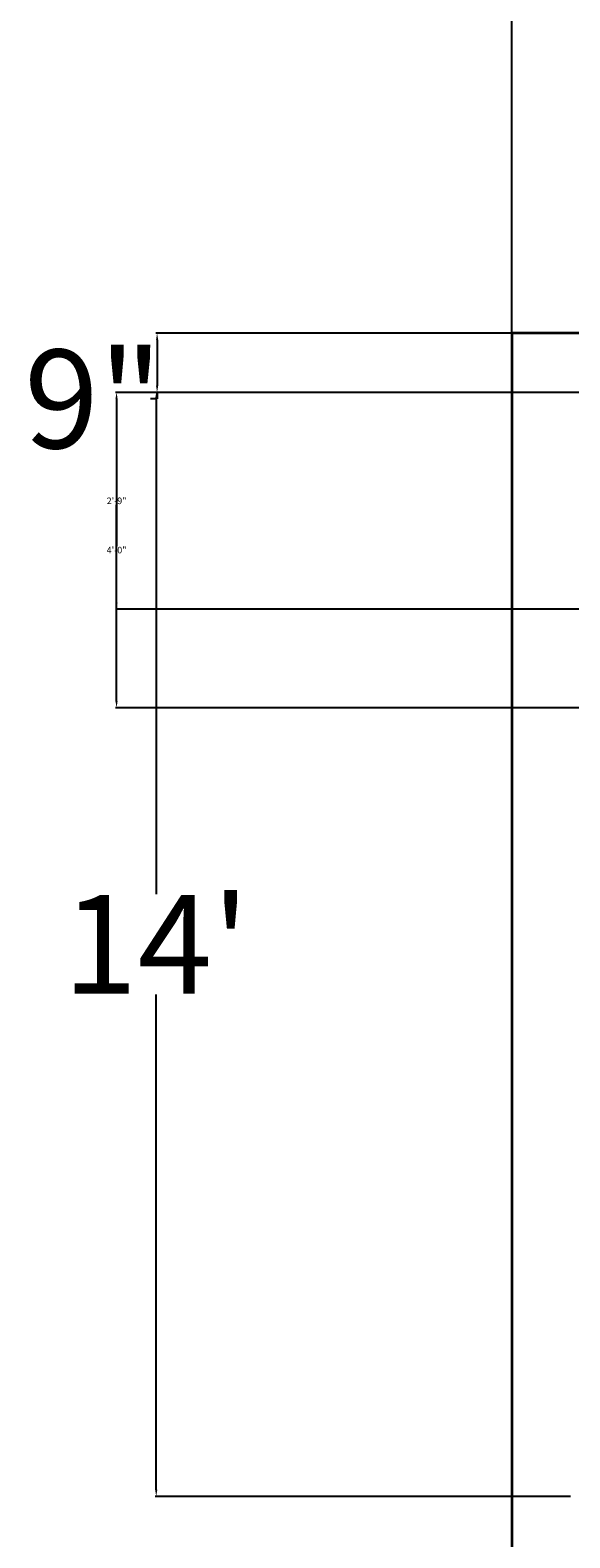
# Model space of a CAD drawing. Units: inches. Extents: x 371 to 1095, y -45 to 1219.
# Tile 14 of 18: x 419 to 502, y 799 to 1028. Entities that reach past the tile are written whole.
import ezdxf

# ---------------------------------------------------------------- set-up
doc = ezdxf.new("R2010")
doc.units = ezdxf.units.IN
doc.header["$MEASUREMENT"] = 0
doc.layers.add('A-ANNO-DIMS', color=2, linetype='Continuous', lineweight=18)
doc.layers.add('A-WALL', color=40, linetype='Continuous', lineweight=35)
doc.styles.get("Standard").update_dxf_attribs({"font": 'arial.ttf'})
doc.dimstyles.get("Standard").update_dxf_attribs({"dimtxt": 1, "dimasz": 1, "dimexe": 0.18, "dimexo": 0.0625, "dimgap": 0.09, "dimtad": 0, "dimtih": 1, "dimtoh": 1, "dimdec": 0, "dimzin": 0, "dimdsep": 46, "dimlunit": 3, "dimtxsty": 'Standard', "dimcen": 0.09, "dimadec": 0, "dimazin": 0, "dimtfac": 1, "dimtdec": 0, "dimtofl": 0, "dimtmove": 0, "dimatfit": 3, "dimfxl": 1, "dimtolj": 1, "dimtzin": 0, "dimarcsym": 0})

# ---------------------------------------------------------------- blocks, each defined once
blk = doc.blocks.new('*D8')
at = {"layer": 'A-ANNO-DIMS', "color": 0, "lineweight": -2, "transparency": 16777216}
for p, q in [((501.75, 973.03), (438.47, 973.03)), ((438.65, 972.03), (438.65, 896.65)), ((438.65, 806.03), (438.65, 881.4)), ((501.75, 805.03), (438.47, 805.03))]:
    blk.add_line(p, q, dxfattribs=at)
at = {"layer": 'A-ANNO-DIMS', "color": 0, "transparency": 16777216}
for points in [[(438.48, 972.03), (438.82, 972.03), (438.65, 973.03)], [(438.48, 806.03), (438.82, 806.03), (438.65, 805.03)]]:
    blk.add_solid(points, dxfattribs=at)
at = {"layer": 'Defpoints', "color": 0, "transparency": 16777216}
for p in [(501.81, 973.03), (438.65, 805.03), (501.81, 805.03)]:
    blk.add_point(p, dxfattribs=at)
at = {"layer": 'A-ANNO-DIMS', "color": 0, "transparency": 16777216, "insert": (438.65, 889.03), "char_height": 1, "attachment_point": 5}
blk.add_mtext("\\A1;{\\H15x;14'}", dxfattribs=at)
blk = doc.blocks.new('*D19')
at = {"layer": 'A-ANNO-DIMS', "color": 0, "lineweight": -2, "transparency": 16777216}
for p, q in [((501.75, 982.03), (438.6, 982.03)), ((438.78, 981.03), (438.78, 974.03)), ((501.75, 973.03), (438.6, 973.03)), ((438.78, 973.03), (438.78, 972.03)), ((438.78, 972.03), (437.78, 972.03))]:
    blk.add_line(p, q, dxfattribs=at)
at = {"layer": 'A-ANNO-DIMS', "color": 0, "transparency": 16777216}
for points in [[(438.62, 981.03), (438.95, 981.03), (438.78, 982.03)], [(438.62, 974.03), (438.95, 974.03), (438.78, 973.03)]]:
    blk.add_solid(points, dxfattribs=at)
at = {"layer": 'Defpoints', "color": 0, "transparency": 16777216}
for p in [(501.81, 982.03), (438.78, 973.03), (501.81, 973.03)]:
    blk.add_point(p, dxfattribs=at)
at = {"layer": 'A-ANNO-DIMS', "color": 0, "transparency": 16777216, "insert": (429.07, 972.03), "char_height": 1, "attachment_point": 5}
blk.add_mtext('\\A1;{\\H15x;9"}', dxfattribs=at)
blk = doc.blocks.new('*D50')
at = {"layer": 'A-ANNO-DIMS', "color": 0, "lineweight": -2, "transparency": 16777216}
for p, q in [((492.81, 982.09), (492.81, 1093.41)), ((493.81, 1093.23), (760.98, 1093.23)), ((1031.81, 1093.23), (764.64, 1093.23)), ((1032.81, 982.09), (1032.81, 1093.41))]:
    blk.add_line(p, q, dxfattribs=at)
at = {"layer": 'A-ANNO-DIMS', "color": 0, "transparency": 16777216}
for points in [[(493.81, 1093.39), (493.81, 1093.06), (492.81, 1093.23)], [(1031.81, 1093.39), (1031.81, 1093.06), (1032.81, 1093.23)]]:
    blk.add_solid(points, dxfattribs=at)
at = {"layer": 'Defpoints', "color": 0, "transparency": 16777216}
for p in [(1032.81, 1093.23), (492.81, 982.03), (1032.81, 982.03)]:
    blk.add_point(p, dxfattribs=at)
at = {"layer": 'A-ANNO-DIMS', "color": 0, "transparency": 16777216, "insert": (762.81, 1093.23), "char_height": 1, "attachment_point": 5}
blk.add_mtext('\\A1;45\'-0"', dxfattribs=at)
blk = doc.blocks.new('*D55')
at = {"layer": 'A-ANNO-DIMS', "color": 0, "lineweight": -2, "transparency": 16777216}
for p, q in [((603.75, 973.03), (432.43, 973.03)), ((432.61, 972.03), (432.61, 949.63)), ((432.61, 926.03), (432.61, 948.42)), ((603.75, 925.03), (432.43, 925.03))]:
    blk.add_line(p, q, dxfattribs=at)
at = {"layer": 'A-ANNO-DIMS', "color": 0, "transparency": 16777216}
for points in [[(432.44, 972.03), (432.77, 972.03), (432.61, 973.03)], [(432.44, 926.03), (432.77, 926.03), (432.61, 925.03)]]:
    blk.add_solid(points, dxfattribs=at)
at = {"layer": 'Defpoints', "color": 0, "transparency": 16777216}
for p in [(432.61, 973.03), (603.81, 973.03), (603.81, 925.03)]:
    blk.add_point(p, dxfattribs=at)
at = {"layer": 'A-ANNO-DIMS', "color": 0, "transparency": 16777216, "insert": (432.61, 949.03), "char_height": 1, "attachment_point": 5}
blk.add_mtext('\\A1;4\'-0"', dxfattribs=at)
blk = doc.blocks.new('*D59')
at = {"layer": 'A-ANNO-DIMS', "color": 0, "lineweight": -2, "transparency": 16777216}
for p, q in [((626.67, 973.03), (432.43, 973.03)), ((432.61, 972.03), (432.61, 957.13)), ((432.61, 941.03), (432.61, 955.92)), ((637.17, 940.03), (432.43, 940.03))]:
    blk.add_line(p, q, dxfattribs=at)
at = {"layer": 'A-ANNO-DIMS', "color": 0, "transparency": 16777216}
for points in [[(432.44, 972.03), (432.77, 972.03), (432.61, 973.03)], [(432.44, 941.03), (432.77, 941.03), (432.61, 940.03)]]:
    blk.add_solid(points, dxfattribs=at)
at = {"layer": 'Defpoints', "color": 0, "transparency": 16777216}
for p in [(432.61, 973.03), (626.74, 973.03), (637.24, 940.03)]:
    blk.add_point(p, dxfattribs=at)
at = {"layer": 'A-ANNO-DIMS', "color": 0, "transparency": 16777216, "insert": (432.61, 956.53), "char_height": 1, "attachment_point": 5}
blk.add_mtext('\\A1;2\'-9"', dxfattribs=at)

msp = doc.modelspace()

# ---------------------------------------------------------------- linework, layer by layer
at = {"layer": 'A-WALL'}
for p, q in [((1032.81, 982.03), (492.81, 982.03)), ((492.81, 982.03), (492.81, 82.03))]:
    msp.add_line(p, q, dxfattribs=at)

# ---------------------------------------------------------------- dimensions: what is measured, and where the dimension line sits
at = {"layer": 'A-ANNO-DIMS'}
dim = msp.add_linear_dim(base=(1032.81, 1093.23), p1=(492.81, 982.03), p2=(1032.81, 982.03), dimstyle='Standard', override={"dimdec": 1, "dimlfac": 1, "dimrnd": 0, "dimzin": 1, "dimdsep": 46, "dimlunit": 4, "dimfrac": 2}, dxfattribs=at)
dim.commit()
dim.dimension.update_dxf_attribs({"geometry": '*D50', "text_midpoint": (762.81, 1093.23)})
for base, p1, p2, picture, middle in [((438.78, 973.03), (501.81, 982.03), (501.81, 973.03), '*D19', (429.07, 972.03)), ((438.65, 805.03), (501.81, 973.03), (501.81, 805.03), '*D8', (438.65, 889.03))]:
    dim = msp.add_linear_dim(base=base, p1=p1, p2=p2, angle=90, text='{\\H15x;<>}', dimstyle='Standard', override={"dimclrd": 0, "dimclre": 0, "dimclrt": 0}, dxfattribs=at)
    dim.commit()
    dim.dimension.update_dxf_attribs({"geometry": picture, "text_midpoint": middle})
for p1, p2, picture, middle in [((603.81, 925.03), (603.81, 973.03), '*D55', (432.61, 949.03)), ((637.24, 940.03), (626.74, 973.03), '*D59', (432.61, 956.53))]:
    dim = msp.add_linear_dim(base=(432.61, 973.03), p1=p1, p2=p2, angle=90, dimstyle='Standard', override={"dimdec": 1, "dimlfac": 1, "dimrnd": 0, "dimzin": 1, "dimdsep": 46, "dimlunit": 4, "dimfrac": 2}, dxfattribs=at)
    dim.commit()
    dim.dimension.update_dxf_attribs({"geometry": picture, "text_midpoint": middle})

doc.saveas('drawing.dxf')
